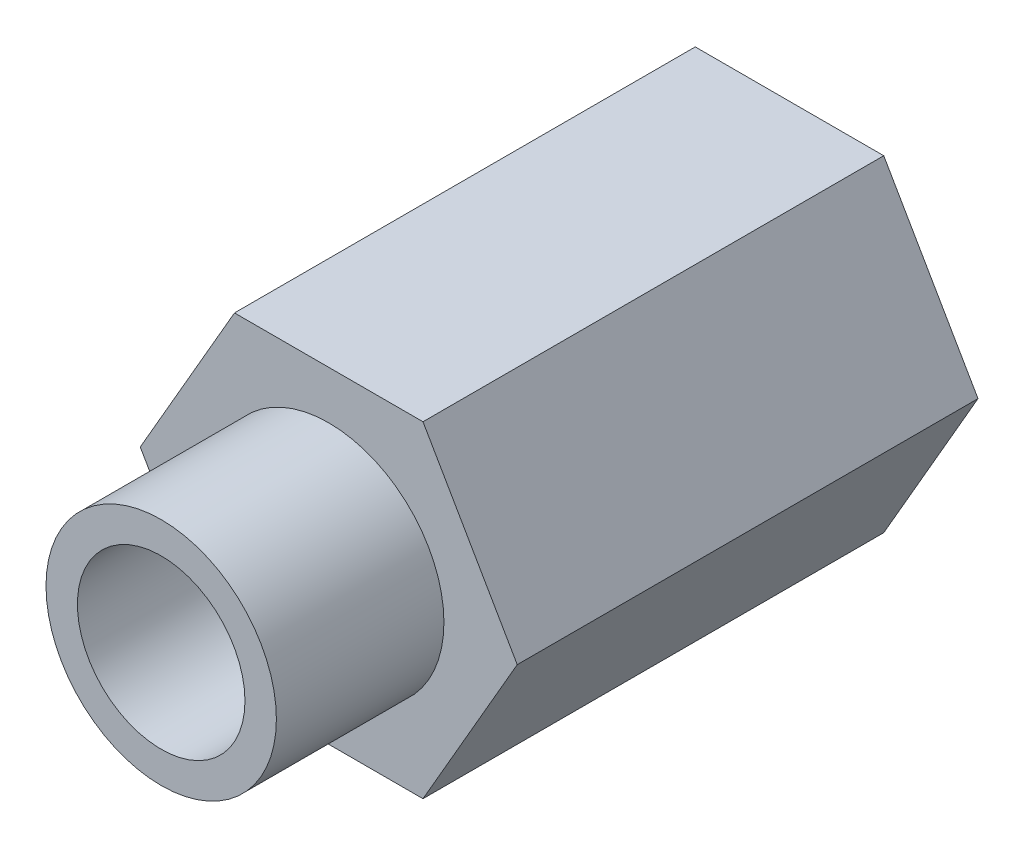
SolidWorks part; units mm, degrees
material "Plain Carbon Steel"
ref_plane "Front Plane" through (0, 0, 0) normal (0, 0, 1) x (1, 0, 0)
ref_plane "Top Plane" through (0, 0, 0) normal (0, 1, 0) x (1, 0, 0)
ref_plane "Right Plane" through (0, 0, 0) normal (1, 0, 0) x (0, 0, -1)
sketch "Hex Profile Sketch" plane through (0, 0, 0) normal (0, 0, 1) x (1, 0, 0)
  line L1 (9, 0) -> (4.5, 7.7942)
  line L2 (4.5, 7.7942) -> (-4.5, 7.7942)
  line L3 (-4.5, 7.7942) -> (-9, 0)
  line L4 (-9, 0) -> (-4.5, -7.7942)
  line L5 (-4.5, -7.7942) -> (4.5, -7.7942)
  line L6 (4.5, -7.7942) -> (9, 0)
  circle A0 centre (0, 0) radius 9 construction
  dimension "D1" = 9
extrude "Hex Body 22mm" add sketch "Hex Profile Sketch" along normal blind 22
sketch "Spigot Sketch Ø11" plane through (0, 0, 22) normal (0, 0, 1) x (1, 0, 0)
  circle A0 centre (0, 0) radius 5.5
  dimension "D1" = 11
extrude "Spigot Ø11x8" add sketch "Spigot Sketch Ø11" along normal blind 8
sketch "Spigot Bore Sketch" plane through (0, 0, 30) normal (0, 0, 1) x (1, 0, 0)
  circle A0 centre (0, 0) radius 4
  dimension "D1" = 8
extrude "Spigot Through Bore" cut sketch "Spigot Bore Sketch" against normal through all
sketch "Hex Bore Sketch Ø12" plane through (0, 0, 0) normal (0, 0, -1) x (-1, 0, 0)
  circle A0 centre (0, 0) radius 6
  dimension "D1" = 12
extrude "Hex Bore Ø12x15" cut sketch "Hex Bore Sketch Ø12" against normal blind 15
